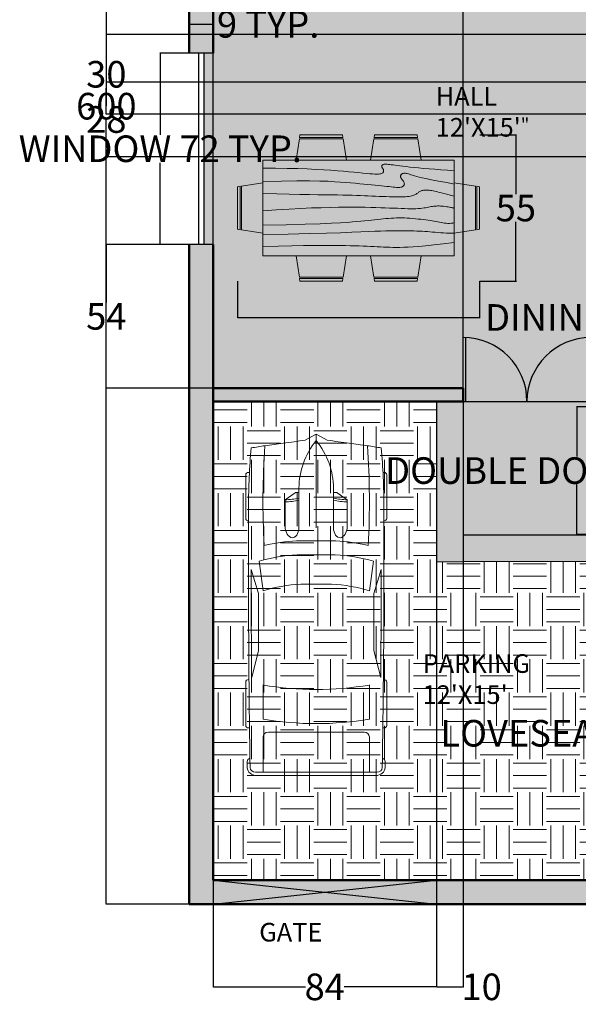
# Model space of a CAD drawing. Units: inches. Extents: x 77 to 548, y 631 to 1307.
# Tile 1 of 4: x 77 to 287, y 631 to 1001. Entities that reach past the tile are written whole.
import ezdxf

# ---------------------------------------------------------------- set-up
doc = ezdxf.new("R2010")
doc.units = ezdxf.units.IN
doc.header["$MEASUREMENT"] = 0
for name, color, linetype, lineweight in [('A-ANNO-DIMS', 2, 'Continuous', 18), ('A-ANNO-TEXT', 7, 'Continuous', 18), ('A-AREA-IDEN', 7, 'Continuous', 18), ('A-FLOR-STRS', 7, 'Continuous', 25), ('A-SITE-GATE', 7, 'Continuous', 25), ('A-WALL', 7, 'Continuous', 50), ('CAR', 7, 'Continuous', 13), ('DOORS', 4, 'Continuous', 25), ('FURNITURE', 34, 'Continuous', 18), ('WINDOW', 6, 'Continuous', 25)]:
    doc.layers.add(name, color=color, linetype=linetype, lineweight=lineweight)
for name, color, linetype, lineweight, true_color in [('A-FLOR-PATT', 254, 'Continuous', 13, 0xd7ebd2), ('A-WALL-PATT', 252, 'Continuous', 13, 0x939598), ('C-PVMT-PATT', 31, 'Continuous', 13, 0xfecc66)]:
    doc.layers.add(name, color=color, linetype=linetype, lineweight=lineweight, true_color=true_color)
doc.styles.get("Standard").update_dxf_attribs({"font": 'arial.ttf'})
doc.dimstyles.get("Standard").update_dxf_attribs({"dimtxt": 10, "dimasz": 0.18, "dimexe": 0.18, "dimexo": 0.0625, "dimgap": 0.09, "dimtad": 0, "dimtih": 1, "dimtoh": 1, "dimdec": 0, "dimzin": 0, "dimdsep": 46, "dimlunit": 3, "dimtxsty": 'Standard', "dimcen": 0.09, "dimadec": 0, "dimazin": 0, "dimtfac": 1, "dimtdec": 0, "dimtofl": 0, "dimtmove": 0, "dimatfit": 3, "dimfxl": 1, "dimtolj": 1, "dimtzin": 0, "dimarcsym": 0})

# ---------------------------------------------------------------- blocks, each defined once
blk = doc.blocks.new('*U3')
for p, q in [((46.55, 38.89), (22.35, 38.89)), ((136.7, 38.89), (160.9, 38.89)), ((21.1, 37.41), (21.1, 36.83)), ((47.8, 37.39), (47.8, 37.41)), ((87.99, 31.87), (74.76, 35.92)), ((134.31, 35.6), (119.29, 31.78)), ((135.45, 37.07), (135.45, 37.41)), ((162.15, 37.41), (162.15, 36.77)), ((186.47, -33.5), (186.47, 33.5)), ((188.4, -32.76), (188.4, 32.76)), ((70.03, 31.54), (86.41, 29.35)), ((138.42, 29.35), (157.25, 29.35)), ((186.47, 29.35), (167.01, 29.35)), ((164.52, 26.39), (164.52, -26.39)), ((32.27, 11.63), (36.13, 17.17)), ((36.13, 17.17), (50.94, 17.17)), ((32.12, 9.51), (32.12, 11.15)), ((3.27, 6.13), (0.1, 0.41)), ((29.77, 9.51), (51.68, 9.51)), ((58.92, -10.77), (58.92, 10.77)), ((66.55, -10.53), (66.55, 10.53)), ((82.74, 8.5), (82.74, -8.5)), ((186.47, -10.53), (186.47, 10.53)), ((0, 0), (51.68, 0)), ((0.1, -0.41), (3.27, -6.13)), ((29.77, -9.51), (51.68, -9.51)), ((32.12, -9.51), (32.12, -11.15)), ((32.27, -11.63), (36.13, -17.17)), ((36.13, -17.17), (50.94, -17.17)), ((86.41, -29.35), (70.03, -31.54)), ((87.99, -31.87), (74.76, -35.92)), ((134.31, -35.6), (119.29, -31.78)), ((157.25, -29.35), (138.42, -29.35)), ((167.01, -29.35), (186.47, -29.35)), ((21.1, -37.41), (21.1, -36.83)), ((47.8, -37.39), (47.8, -37.41)), ((135.45, -37.07), (135.45, -37.41)), ((162.15, -37.41), (162.15, -36.77)), ((46.55, -38.89), (22.35, -38.89)), ((136.7, -38.89), (160.9, -38.89))]:
    blk.add_line(p, q)
for centre, major_axis, ratio, start_param, end_param in [((22.35, 37.41), (0, -1.48), 0.842304, 3.141593, 4.712389), ((46.55, 37.41), (0, 1.48), 0.842304, -1.570796, 0), ((136.7, 37.41), (0, -1.48), 0.842304, 3.141593, 4.712389), ((160.9, 37.41), (0, 1.48), 0.842304, -1.570796, 0), ((180.63, 35.84), (0, 2.22), 0.842304, -0.013017, 1.249894), ((64.48, -10556.36), (0, 10595.31), 0.842304, -0.013397, -0.013017), ((266.03, -27.52), (0, 313.31), 0.842304, 1.367076, 1.39176), ((41.19, -490.86), (0, 528.23), 0.842304, 0.00281, 0.075598), ((64.48, -10555.62), (0, 10593.03), 0.842304, -0.013397, 0.002797), ((64.48, -10555.62), (0, -10591.55), 0.842304, 3.133765, 3.140441), ((183.98, 33.5), (0, -2.96), 0.842304, 1.570796, 3.128196), ((183.98, 32.76), (0, -5.25), 0.842304, 1.570796, 3.128196), ((259.18, -27.52), (0, -305.3), 0.842304, 4.528606, 4.561838), ((37.47, -593.96), (0, -623.33), 0.842304, 3.096046, 3.200911), ((134.4, 5.39), (0, -89.78), 0.842304, 4.449482, 4.652344), ((135.29, 5.39), (0, 81.77), 0.842304, 1.245306, 1.50788), ((149.6, 2.8), (0, -79.58), 0.842304, 4.372215, 4.640744), ((95.79, -3666.35), (0, -3698.24), 0.842304, 3.134049, 3.144098), ((17.08, 0), (0, 147.02), 0.842304, 4.511394, 4.913384), ((35.91, 0), (0, 147.02), 0.842304, 4.511394, 4.913384), ((167.01, 26.39), (0, 2.96), 0.842304, 0, 1.570796), ((-204.49, 52.4), (0, -250.96), 0.842304, 1.385369, 1.434372), ((13.04, 17.01), (0, 27.42), 0.842304, 4.435146, 4.718221), ((14.2, 17.01), (0, 27.42), 0.842304, 4.435146, 4.718221), ((50.79, 13.34), (6.34, -0.36), 0.603834, -1.395552, 1.581315), ((32.75, 11.15), (0, 0.74), 0.842304, 0.879714, 1.570796), ((29.77, -46.66), (0, 56.17), 0.842304, 0, 0.590319), ((0.62, 0), (0, -0.74), 0.842304, 4.131459, 5.293319), ((29.77, 46.66), (0, 56.17), 0.842304, 2.551274, 3.141593), ((-204.49, -52.4), (0, 250.96), 0.842304, -1.434372, -1.385369), ((13.04, -17.01), (0, -27.42), 0.842304, 1.564964, 1.848039), ((14.2, -17.01), (0, -27.42), 0.842304, 1.564964, 1.848039), ((134.4, -5.39), (0, -89.78), 0.842304, -1.510751, -1.307889), ((135.29, -5.39), (0, -81.77), 0.842304, -1.50788, -1.245306), ((149.6, -2.8), (0, -79.58), 0.842304, -1.499151, -1.230623), ((32.75, -11.15), (0, -0.74), 0.842304, 4.712389, 5.403472), ((259.18, 27.52), (0, 305.3), 0.842304, 1.721348, 1.754579), ((167.01, -26.39), (0, -2.96), 0.842304, 4.712389, 6.283185), ((266.03, 27.52), (0, 313.31), 0.842304, 1.749832, 1.774517), ((37.47, 593.96), (0, -623.33), 0.842304, -0.059319, 0.045547), ((95.79, 3666.35), (0, -3698.24), 0.842304, -0.002505, 0.007544), ((41.19, 490.86), (0, -528.23), 0.842304, -0.075598, -0.00281), ((22.35, -37.41), (0, 1.48), 0.842304, 1.570796, 3.141593), ((64.48, 10555.62), (0, 10593.03), 0.842304, 3.138796, 3.15499), ((46.55, -37.41), (0, -1.48), 0.842304, 0, 1.570796), ((64.48, 10555.62), (0, -10591.55), 0.842304, 0.001152, 0.007828), ((136.7, -37.41), (0, -1.48), 0.842304, -1.570796, 0), ((160.9, -37.41), (0, 1.48), 0.842304, 3.141593, 4.712389), ((180.63, -35.84), (0, -2.22), 0.842304, -1.249894, 0.013017), ((64.48, 10556.36), (0, 10595.31), 0.842304, 3.15461, 3.15499), ((183.98, -33.5), (0, 2.96), 0.842304, 3.15499, 4.712389), ((183.98, -32.76), (0, -5.25), 0.842304, 0.013397, 1.570796)]:
    blk.add_ellipse(centre, major_axis=major_axis, ratio=ratio, start_param=start_param, end_param=end_param)
at = {"extrusion": (0, 0, -1)}
blk.add_ellipse((50.79, -13.34), major_axis=(6.34, 0.36), ratio=0.603834, start_param=-1.395552, end_param=1.581315, dxfattribs=at)
blk = doc.blocks.new('Dining Set - 36 x 72 in.')
for p, q in [((-22.2343, 26.00059), (-23.4847, 17.99762)), ((-22.2304, 26), (-5.7608, 26)), ((-22, 27.5), (-22.1562, 26.50042)), ((-5.8416, 26.5), (-22.1534, 26.5)), ((-22, 27.5), (-6, 27.5)), ((-5.8437, 26.49966), (-6, 27.5)), ((-4.5152, 17.99762), (-5.7655, 25.99926)), ((5.7657, 26.00059), (4.5153, 17.99762)), ((5.7696, 26), (22.2392, 26)), ((6, 27.5), (5.8438, 26.50042)), ((22.1584, 26.5), (5.8466, 26.5)), ((6, 27.5), (22, 27.5)), ((22.1563, 26.49966), (22, 27.5)), ((23.4848, 17.99762), (22.2345, 25.99926)), ((36, 18), (-36, 18)), ((-36, 18), (-36, -18)), ((36, -18), (36, 18)), ((-45.5, 8), (-44.5004, 8.15617)), ((-45.5, 8), (-45.5, -8)), ((-44.5, -8.15843), (-44.5, 8.15338)), ((-44.0006, 8.23428), (-35.9976, 9.48474)), ((-44, 8.23041), (-44, -8.23915)), ((44.0006, 8.23428), (35.9976, 9.48474)), ((44, 8.23041), (44, -8.23915)), ((44.5, -8.15843), (44.5, 8.15338)), ((45.5, 8), (44.5005, 8.15617)), ((45.5, 8), (45.5, -8)), ((-44.4997, -8.15631), (-45.5, -8)), ((-35.9976, -9.48476), (-43.9993, -8.2345)), ((35.9976, -9.48476), (43.9993, -8.2345)), ((44.4997, -8.15631), (45.5, -8)), ((-36, -18), (36, -18)), ((-22.2343, -26.0006), (-23.4847, -17.99762)), ((-4.5152, -17.99762), (-5.7655, -25.99928)), ((5.7657, -26.0006), (4.5153, -17.99762)), ((23.4848, -17.99762), (22.2345, -25.99928)), ((-22.2304, -26), (-5.7608, -26)), ((-22, -27.5), (-22.1562, -26.50044)), ((-5.8416, -26.5), (-22.1534, -26.5)), ((-22, -27.5), (-6, -27.5)), ((-5.8437, -26.49967), (-6, -27.5)), ((5.7696, -26), (22.2392, -26)), ((6, -27.5), (5.8438, -26.50044)), ((22.1584, -26.5), (5.8466, -26.5)), ((6, -27.5), (22, -27.5)), ((22.1563, -26.49967), (22, -27.5))]:
    blk.add_line(p, q)
for points in [[(-36, 15), (-31.1772, 14.97754), (-26.8079, 14.91406), (-22.8538, 14.81543), (-19.276, 14.6875), (-16.0362, 14.53613), (-13.0957, 14.36718), (-10.4159, 14.18652), (-7.9583, 14), (-5.6904, 13.81315), (-3.6035, 13.63021), (-1.6954, 13.45508), (0.0365, 13.29166), (1.5945, 13.14388), (2.9811, 13.01562), (4.1988, 12.9108), (5.25, 12.83333), (6.1393, 12.78613), (6.8802, 12.76823), (7.4883, 12.77767), (7.9792, 12.8125), (8.3685, 12.87077), (8.6719, 12.95052), (8.9049, 13.0498), (9.0833, 13.16666), (9.2205, 13.29899), (9.3216, 13.44401), (9.3895, 13.59879), (9.4271, 13.76041), (9.4373, 13.92594), (9.4232, 14.09245), (9.3875, 14.257), (9.3333, 14.41666), (9.2638, 14.56917), (9.1836, 14.71484), (9.0975, 14.85465), (9.0104, 14.98958), (8.9272, 15.1206), (8.8529, 15.2487), (8.7922, 15.37483), (8.75, 15.5), (8.7305, 15.62467), (8.7344, 15.74739), (8.7617, 15.86621), (8.8125, 15.97916), (8.8867, 16.08431), (8.9844, 16.17968), (9.1055, 16.26334), (9.25, 16.33333), (9.4189, 16.38802), (9.6172, 16.42708), (9.8506, 16.45052), (10.125, 16.45833), (10.4463, 16.45052), (10.8203, 16.42708), (11.2529, 16.38802), (11.75, 16.33333), (12.3184, 16.26318), (12.9694, 16.17838), (13.7151, 16.07991), (14.5677, 15.96875), (15.5395, 15.84586), (16.6426, 15.71224), (17.8893, 15.56884), (19.2917, 15.41666), (20.859, 15.25667), (22.5879, 15.08984), (24.4721, 14.91715), (26.5052, 14.73958), (28.6809, 14.5581), (30.9929, 14.3737), (33.4347, 14.18733), (36, 14)], [(-36, 10), (-28.9766, 10.14274), (-23.1725, 10.20442), (-18.4241, 10.19775), (-14.5677, 10.13541), (-11.4399, 10.03011), (-8.877, 9.89453), (-6.7154, 9.74137), (-4.7917, 9.58333), (-2.9698, 9.43082), (-1.2246, 9.28515), (0.4415, 9.14534), (2.026, 9.01041), (3.5266, 8.87939), (4.9408, 8.7513), (6.266, 8.62516), (7.5, 8.5), (8.6411, 8.37549), (9.6914, 8.2539), (10.6538, 8.13818), (11.5312, 8.03125), (12.3267, 7.93603), (13.043, 7.85547), (13.6831, 7.79248), (14.25, 7.75), (14.7471, 7.7303), (15.1797, 7.73307), (15.5537, 7.75732), (15.875, 7.80208), (16.1494, 7.86637), (16.3828, 7.94922), (16.5811, 8.04964), (16.75, 8.16666), (16.8944, 8.29915), (17.0143, 8.44531), (17.1089, 8.60319), (17.1771, 8.77083), (17.218, 8.94629), (17.2305, 9.1276), (17.2137, 9.31282), (17.1667, 9.5), (17.0895, 9.6875), (16.987, 9.875), (16.8649, 10.0625), (16.7292, 10.25), (16.5856, 10.4375), (16.4401, 10.625), (16.2985, 10.8125), (16.1667, 11), (16.05, 11.18733), (15.9518, 11.3737), (15.8752, 11.5581), (15.8229, 11.73958), (15.798, 11.91715), (15.8034, 12.08984), (15.842, 12.25667), (15.9167, 12.41666), (16.0295, 12.56836), (16.1784, 12.70833), (16.3605, 12.83268), (16.5729, 12.9375), (16.8127, 13.01888), (17.0768, 13.07291), (17.3625, 13.0957), (17.6667, 13.08333), (17.9894, 13.03312), (18.3418, 12.94726), (18.7382, 12.82918), (19.1927, 12.68229), (19.7195, 12.51001), (20.3327, 12.31575), (21.0465, 12.10294), (21.875, 11.875), (22.8357, 11.63354), (23.959, 11.37304), (25.2786, 11.08618), (26.8282, 10.76562), (28.6414, 10.40405), (30.752, 9.99414), (33.1936, 9.52856), (36, 9)], [(-36, 5.5), (-30.7157, 5.3348), (-26.069, 5.20963), (-21.9946, 5.11767), (-18.4271, 5.05208), (-15.3009, 5.00602), (-12.5508, 4.97265), (-10.1112, 4.94515), (-7.9167, 4.91666), (-5.909, 4.88167), (-4.0586, 4.83984), (-2.3429, 4.79215), (-0.7396, 4.73958), (0.7739, 4.6831), (2.22, 4.6237), (3.6213, 4.56233), (5, 4.5), (6.373, 4.43782), (7.7344, 4.3776), (9.0723, 4.32129), (10.375, 4.27083), (11.6309, 4.22819), (12.8281, 4.19531), (13.9551, 4.17415), (15, 4.16666), (15.954, 4.17448), (16.819, 4.19791), (17.6001, 4.23698), (18.3021, 4.29166), (18.9299, 4.36198), (19.4883, 4.44791), (19.9823, 4.54948), (20.4167, 4.66666), (20.7969, 4.79899), (21.1302, 4.94401), (21.4245, 5.09879), (21.6875, 5.26041), (21.9271, 5.42594), (22.1511, 5.59245), (22.3672, 5.757), (22.5834, 5.91666), (22.8065, 6.06868), (23.0404, 6.21093), (23.2879, 6.34147), (23.5521, 6.45833), (23.8358, 6.55957), (24.142, 6.64323), (24.4735, 6.70735), (24.8334, 6.75), (25.2235, 6.76969), (25.642, 6.76692), (26.0858, 6.74267), (26.5521, 6.69791), (27.0379, 6.63362), (27.5404, 6.55078), (28.0565, 6.45036), (28.5834, 6.33333), (29.1242, 6.19987), (29.7071, 6.04687), (30.3661, 5.87044), (31.1354, 5.66666), (32.0493, 5.43164), (33.142, 5.16146), (34.4475, 4.85221), (36, 4.5)], [(-36, -1), (-30.7915, -0.6591), (-26.0195, -0.38216), (-21.6519, -0.16284), (-17.6563, 0.00521), (-14.0005, 0.12833), (-10.6523, 0.21289), (-7.5796, 0.26522), (-4.75, 0.29166), (-2.134, 0.29793), (0.2878, 0.28711), (2.5317, 0.26163), (4.6146, 0.22396), (6.5529, 0.17651), (8.3633, 0.12174), (10.0623, 0.06209), (11.6667, 0), (13.1899, -0.06201), (14.6341, -0.1211), (15.9982, -0.17432), (17.2813, -0.21875), (18.4823, -0.25147), (19.6003, -0.26953), (20.6343, -0.27002), (21.5834, -0.25), (22.4481, -0.20768), (23.2357, -0.14584), (23.9549, -0.06836), (24.6146, 0.02083), (25.2235, 0.11784), (25.7904, 0.21875), (26.3241, 0.31966), (26.8334, 0.41666), (27.3265, 0.50618), (27.8099, 0.58593), (28.2894, 0.65397), (28.7709, 0.70833), (29.2601, 0.74707), (29.763, 0.76823), (30.2855, 0.76985), (30.8334, 0.75), (31.4088, 0.70784), (31.9994, 0.64713), (32.589, 0.57275), (33.1615, 0.48958), (33.7008, 0.4025), (34.1908, 0.3164), (34.6153, 0.23616), (34.9584, 0.16666), (35.2099, 0.11165), (35.3848, 0.07031), (35.504, 0.04069), (35.5886, 0.02083), (35.6594, 0.00879), (35.7377, 0.0026), (35.8442, 0.00032), (36, 0)], [(-36, -6.5), (-27.1843, -6.31267), (-20.084, -6.1263), (-14.469, -5.9419), (-10.1094, -5.76042), (-6.7752, -5.58285), (-4.2363, -5.41016), (-2.2629, -5.24333), (-0.625, -5.08334), (0.8708, -4.93099), (2.2715, -4.78646), (3.5872, -4.64974), (4.8281, -4.52084), (6.0046, -4.39974), (7.127, -4.28646), (8.2053, -4.18099), (9.25, -4.08334), (10.2705, -3.99382), (11.2734, -3.91407), (12.2647, -3.84603), (13.25, -3.79167), (14.2354, -3.75293), (15.2266, -3.73177), (16.2295, -3.73015), (17.25, -3.75), (18.2912, -3.79248), (19.3451, -3.85547), (20.4009, -3.93604), (21.4479, -4.03125), (22.4754, -4.13819), (23.4727, -4.25391), (24.4289, -4.37549), (25.3334, -4.5), (26.1785, -4.62492), (26.9694, -4.74935), (27.7145, -4.87281), (28.4219, -4.99479), (29.1, -5.11483), (29.7572, -5.23242), (30.4016, -5.34709), (31.0417, -5.45834), (31.6837, -5.56437), (32.3262, -5.65821), (32.9658, -5.73153), (33.599, -5.77604), (34.2224, -5.78345), (34.8327, -5.74545), (35.4264, -5.65373), (36, -5.5)], [(-36, -10), (-26.4022, -9.81299), (-18.4675, -9.62891), (-11.9839, -9.45069), (-6.7396, -9.28125), (-2.5226, -9.12354), (0.8789, -8.98047), (3.6769, -8.85498), (6.0833, -8.75), (8.2767, -8.66765), (10.3021, -8.60677), (12.1712, -8.56543), (13.8958, -8.54167), (15.4876, -8.53353), (16.9583, -8.53907), (18.3197, -8.55632), (19.5834, -8.58334), (20.7616, -8.61841), (21.8685, -8.66081), (22.9188, -8.71004), (23.9271, -8.76563), (24.9081, -8.82707), (25.8763, -8.89388), (26.8465, -8.96558), (27.8334, -9.04167), (28.8474, -9.12118), (29.8828, -9.20117), (30.93, -9.27824), (31.9792, -9.34896), (33.0205, -9.40991), (34.0443, -9.45768), (35.0407, -9.48885), (36, -9.5)], [(-36, -14.5), (-30.0881, -14.33513), (-25.0332, -14.21224), (-20.7312, -14.12647), (-17.0781, -14.07292), (-13.97, -14.04671), (-11.3027, -14.04297), (-8.9724, -14.05681), (-6.875, -14.08334), (-4.9224, -14.11833), (-3.0905, -14.16016), (-1.3709, -14.20785), (0.2448, -14.26042), (1.7647, -14.3169), (3.1973, -14.3763), (4.5507, -14.43767), (5.8333, -14.5), (7.0554, -14.5621), (8.235, -14.62175), (9.3922, -14.67652), (10.5469, -14.72396), (11.7192, -14.76164), (12.929, -14.78711), (14.1965, -14.79794), (15.5417, -14.79167), (16.9933, -14.76424), (18.6152, -14.70508), (20.4804, -14.60197), (22.6615, -14.44271), (25.2312, -14.21509), (28.2624, -13.9069), (31.8277, -13.50594), (36, -13)]]:
    blk.add_lwpolyline(points)
blk = doc.blocks.new('WINDOW-72')
for p, q in [((9, 72), (0, 72)), ((3.5, 72), (3.5, 0)), ((5.5, 72), (5.5, 0)), ((9, 0), (0, 0))]:
    blk.add_line(p, q)
blk = doc.blocks.new('DOOR-DOUBLE-48')
for p, q in [((0, 0), (0, 24)), ((1, 0), (1, 23.98)), ((47, 0), (47, 23.98)), ((48, 0), (48, 24)), ((0, 0), (1, 0)), ((47, 0), (48, 0))]:
    blk.add_line(p, q)
for centre, start, end in [((0, 0), 0, 90), ((48, 0), 90, 180)]:
    blk.add_arc(centre, 24, start, end)
blk = doc.blocks.new('*D24')
at = {"layer": 'A-ANNO-DIMS', "color": 0, "lineweight": -2, "transparency": 16777216}
for p, q in [((140.6, 988.89), (129.68, 988.89)), ((129.86, 988.71), (129.86, 958.15)), ((129.86, 917.07), (129.86, 947.62)), ((140.6, 916.89), (129.68, 916.89))]:
    blk.add_line(p, q, dxfattribs=at)
at = {"layer": 'A-ANNO-DIMS', "color": 0, "transparency": 16777216}
for points in [[(129.83, 988.71), (129.89, 988.71), (129.86, 988.89)], [(129.83, 917.07), (129.89, 917.07), (129.86, 916.89)]]:
    blk.add_solid(points, dxfattribs=at)
at = {"layer": 'Defpoints', "color": 0, "transparency": 16777216}
for p in [(129.86, 988.89), (140.66, 988.89), (140.66, 916.89)]:
    blk.add_point(p, dxfattribs=at)
at = {"layer": 'A-ANNO-DIMS', "color": 0, "transparency": 16777216, "insert": (129.86, 952.89), "char_height": 10, "attachment_point": 5}
blk.add_mtext('\\A1;WINDOW 72 TYP.', dxfattribs=at)
blk = doc.blocks.new('*D25')
at = {"layer": 'A-ANNO-DIMS', "color": 0, "lineweight": -2, "transparency": 16777216}
for p, q in [((140.66, 988.95), (140.66, 999.87)), ((140.84, 999.69), (149.48, 999.69)), ((149.66, 988.95), (149.66, 999.87)), ((149.66, 999.69), (149.84, 999.69))]:
    blk.add_line(p, q, dxfattribs=at)
at = {"layer": 'A-ANNO-DIMS', "color": 0, "transparency": 16777216}
for points in [[(140.84, 999.72), (140.84, 999.66), (140.66, 999.69)], [(149.48, 999.72), (149.48, 999.66), (149.66, 999.69)]]:
    blk.add_solid(points, dxfattribs=at)
at = {"layer": 'Defpoints', "color": 0, "transparency": 16777216}
for p in [(149.66, 999.69), (140.66, 988.89), (149.66, 988.89)]:
    blk.add_point(p, dxfattribs=at)
at = {"layer": 'A-ANNO-DIMS', "color": 0, "transparency": 16777216, "insert": (170.39, 999.69), "char_height": 10, "attachment_point": 5}
blk.add_mtext('\\A1;9 TYP.', dxfattribs=at)
blk = doc.blocks.new('*D26')
at = {"layer": 'A-ANNO-DIMS', "color": 0, "lineweight": -2, "transparency": 16777216}
for p, q in [((293.6, 855.89), (286.28, 855.89)), ((286.46, 855.71), (286.46, 837.15)), ((286.46, 808.07), (286.46, 826.62)), ((293.6, 807.89), (286.28, 807.89))]:
    blk.add_line(p, q, dxfattribs=at)
at = {"layer": 'A-ANNO-DIMS', "color": 0, "transparency": 16777216}
for points in [[(286.43, 855.71), (286.49, 855.71), (286.46, 855.89)], [(286.43, 808.07), (286.49, 808.07), (286.46, 807.89)]]:
    blk.add_solid(points, dxfattribs=at)
at = {"layer": 'Defpoints', "color": 0, "transparency": 16777216}
for p in [(293.66, 855.89), (286.46, 807.89), (293.66, 807.89)]:
    blk.add_point(p, dxfattribs=at)
at = {"layer": 'A-ANNO-DIMS', "color": 0, "transparency": 16777216, "insert": (286.46, 831.89), "char_height": 10, "attachment_point": 5}
blk.add_mtext('\\A1;DOUBLE DOOR 48 TYP.', dxfattribs=at)
blk = doc.blocks.new('*D36')
at = {"layer": 'A-ANNO-DIMS', "color": 0, "lineweight": -2, "transparency": 16777216}
for p, q in [((158.85, 903.05), (158.85, 889.28)), ((249.85, 903.05), (249.85, 889.28)), ((159.03, 889.46), (249.67, 889.46)), ((249.85, 889.46), (250.03, 889.46))]:
    blk.add_line(p, q, dxfattribs=at)
at = {"layer": 'A-ANNO-DIMS', "color": 0, "transparency": 16777216}
for points in [[(159.03, 889.49), (159.03, 889.43), (158.85, 889.46)], [(249.67, 889.49), (249.67, 889.43), (249.85, 889.46)]]:
    blk.add_solid(points, dxfattribs=at)
at = {"layer": 'Defpoints', "color": 0, "transparency": 16777216}
for p in [(158.85, 903.11), (249.85, 903.11), (249.85, 889.46)]:
    blk.add_point(p, dxfattribs=at)
at = {"layer": 'A-ANNO-DIMS', "color": 0, "transparency": 16777216, "insert": (297.98, 889.46), "char_height": 10, "attachment_point": 5}
blk.add_mtext('\\A1;DINING SET 91', dxfattribs=at)
blk = doc.blocks.new('*D37')
at = {"layer": 'A-ANNO-DIMS', "color": 0, "lineweight": -2, "transparency": 16777216}
for p, q in [((249.91, 958.11), (263.68, 958.11)), ((263.5, 957.93), (263.5, 935.79)), ((263.5, 903.29), (263.5, 925.44)), ((249.91, 903.11), (263.68, 903.11))]:
    blk.add_line(p, q, dxfattribs=at)
at = {"layer": 'A-ANNO-DIMS', "color": 0, "transparency": 16777216}
for points in [[(263.47, 957.93), (263.53, 957.93), (263.5, 958.11)], [(263.47, 903.29), (263.53, 903.29), (263.5, 903.11)]]:
    blk.add_solid(points, dxfattribs=at)
at = {"layer": 'Defpoints', "color": 0, "transparency": 16777216}
for p in [(249.85, 958.11), (263.5, 958.11), (249.85, 903.11)]:
    blk.add_point(p, dxfattribs=at)
at = {"layer": 'A-ANNO-DIMS', "color": 0, "transparency": 16777216, "insert": (263.5, 930.61), "char_height": 10, "attachment_point": 5}
blk.add_mtext('\\A1;55', dxfattribs=at)
blk = doc.blocks.new('*D40')
at = {"layer": 'A-ANNO-DIMS', "color": 0, "lineweight": -2, "transparency": 16777216}
for p, q in [((323.26, 733.13), (323.08, 733.13)), ((323.26, 724.2), (323.26, 733.31)), ((383.08, 733.13), (323.44, 733.13)), ((383.26, 724.2), (383.26, 733.31))]:
    blk.add_line(p, q, dxfattribs=at)
at = {"layer": 'A-ANNO-DIMS', "color": 0, "transparency": 16777216}
for points in [[(323.44, 733.16), (323.44, 733.1), (323.26, 733.13)], [(383.08, 733.16), (383.08, 733.1), (383.26, 733.13)]]:
    blk.add_solid(points, dxfattribs=at)
at = {"layer": 'Defpoints', "color": 0, "transparency": 16777216}
for p in [(323.26, 733.13), (323.26, 724.13), (383.26, 724.13)]:
    blk.add_point(p, dxfattribs=at)
at = {"layer": 'A-ANNO-DIMS', "color": 0, "transparency": 16777216, "insert": (277.25, 733.13), "char_height": 10, "attachment_point": 5}
blk.add_mtext('\\A1;LOVESEAT 60', dxfattribs=at)
blk = doc.blocks.new('*D43')
at = {"layer": 'A-ANNO-DIMS', "color": 0, "lineweight": -2, "transparency": 16777216}
for p, q in [((140.6, 1268.89), (109.38, 1268.89)), ((109.56, 1268.71), (109.56, 974.08)), ((109.56, 669.07), (109.56, 963.69)), ((140.6, 668.89), (109.38, 668.89))]:
    blk.add_line(p, q, dxfattribs=at)
at = {"layer": 'A-ANNO-DIMS', "color": 0, "transparency": 16777216}
for points in [[(109.53, 1268.71), (109.59, 1268.71), (109.56, 1268.89)], [(109.53, 669.07), (109.59, 669.07), (109.56, 668.89)]]:
    blk.add_solid(points, dxfattribs=at)
at = {"layer": 'Defpoints', "color": 0, "transparency": 16777216}
for p in [(109.56, 1268.89), (140.66, 1268.89), (140.66, 668.89)]:
    blk.add_point(p, dxfattribs=at)
at = {"layer": 'A-ANNO-DIMS', "color": 0, "transparency": 16777216, "insert": (109.56, 968.89), "char_height": 10, "attachment_point": 5}
blk.add_mtext('\\A1;600', dxfattribs=at)
blk = doc.blocks.new('*D44')
at = {"layer": 'A-ANNO-DIMS', "color": 0, "lineweight": -2, "transparency": 16777216}
for p, q in [((149.66, 668.83), (149.66, 637.61)), ((233.66, 668.83), (233.66, 637.61)), ((149.84, 637.79), (184.42, 637.79)), ((233.48, 637.79), (198.9, 637.79))]:
    blk.add_line(p, q, dxfattribs=at)
at = {"layer": 'A-ANNO-DIMS', "color": 0, "transparency": 16777216}
for points in [[(149.84, 637.82), (149.84, 637.76), (149.66, 637.79)], [(233.48, 637.82), (233.48, 637.76), (233.66, 637.79)]]:
    blk.add_solid(points, dxfattribs=at)
at = {"layer": 'Defpoints', "color": 0, "transparency": 16777216}
for p in [(149.66, 668.89), (233.66, 668.89), (233.66, 637.79)]:
    blk.add_point(p, dxfattribs=at)
at = {"layer": 'A-ANNO-DIMS', "color": 0, "transparency": 16777216, "insert": (191.66, 637.79), "char_height": 10, "attachment_point": 5}
blk.add_mtext('\\A1;84', dxfattribs=at)
blk = doc.blocks.new('*D47')
at = {"layer": 'A-ANNO-DIMS', "color": 0, "lineweight": -2, "transparency": 16777216}
for p, q in [((140.6, 916.89), (109.38, 916.89)), ((109.56, 916.71), (109.56, 895.06)), ((109.56, 863.07), (109.56, 884.71)), ((149.6, 862.89), (109.38, 862.89))]:
    blk.add_line(p, q, dxfattribs=at)
at = {"layer": 'A-ANNO-DIMS', "color": 0, "transparency": 16777216}
for points in [[(109.53, 916.71), (109.59, 916.71), (109.56, 916.89)], [(109.53, 863.07), (109.59, 863.07), (109.56, 862.89)]]:
    blk.add_solid(points, dxfattribs=at)
at = {"layer": 'Defpoints', "color": 0, "transparency": 16777216}
for p in [(140.66, 916.89), (109.56, 862.89), (149.66, 862.89)]:
    blk.add_point(p, dxfattribs=at)
at = {"layer": 'A-ANNO-DIMS', "color": 0, "transparency": 16777216, "insert": (109.56, 889.89), "char_height": 10, "attachment_point": 5}
blk.add_mtext('\\A1;54', dxfattribs=at)
blk = doc.blocks.new('*D54')
at = {"layer": 'A-ANNO-DIMS', "color": 0, "lineweight": -2, "transparency": 16777216}
for p, q in [((351.6, 995.89), (109.38, 995.89)), ((109.56, 995.71), (109.56, 986.09)), ((109.56, 966.07), (109.56, 975.69)), ((351.6, 965.89), (109.38, 965.89))]:
    blk.add_line(p, q, dxfattribs=at)
at = {"layer": 'A-ANNO-DIMS', "color": 0, "transparency": 16777216}
for points in [[(109.53, 995.71), (109.59, 995.71), (109.56, 995.89)], [(109.53, 966.07), (109.59, 966.07), (109.56, 965.89)]]:
    blk.add_solid(points, dxfattribs=at)
at = {"layer": 'Defpoints', "color": 0, "transparency": 16777216}
for p in [(109.56, 995.89), (351.66, 995.89), (351.66, 965.89)]:
    blk.add_point(p, dxfattribs=at)
at = {"layer": 'A-ANNO-DIMS', "color": 0, "transparency": 16777216, "insert": (109.56, 980.89), "char_height": 10, "attachment_point": 5}
blk.add_mtext('\\A1;30', dxfattribs=at)
blk = doc.blocks.new('*D56')
at = {"layer": 'A-ANNO-DIMS', "color": 0, "lineweight": -2, "transparency": 16777216}
for p, q in [((149.66, 857.95), (149.66, 1300.17)), ((149.84, 1299.99), (189.43, 1299.99)), ((243.48, 1299.99), (203.89, 1299.99)), ((243.66, 857.95), (243.66, 1300.17))]:
    blk.add_line(p, q, dxfattribs=at)
at = {"layer": 'A-ANNO-DIMS', "color": 0, "transparency": 16777216}
for points in [[(149.84, 1300.02), (149.84, 1299.96), (149.66, 1299.99)], [(243.48, 1300.02), (243.48, 1299.96), (243.66, 1299.99)]]:
    blk.add_solid(points, dxfattribs=at)
at = {"layer": 'Defpoints', "color": 0, "transparency": 16777216}
for p in [(243.66, 1299.99), (149.66, 857.89), (243.66, 857.89)]:
    blk.add_point(p, dxfattribs=at)
at = {"layer": 'A-ANNO-DIMS', "color": 0, "transparency": 16777216, "insert": (196.66, 1299.99), "char_height": 10, "attachment_point": 5}
blk.add_mtext('\\A1;94', dxfattribs=at)
blk = doc.blocks.new('*D59')
at = {"layer": 'A-ANNO-DIMS', "color": 0, "lineweight": -2, "transparency": 16777216}
for p, q in [((385.62, 977.89), (109.38, 977.89)), ((109.56, 977.71), (109.56, 969.08)), ((109.56, 950.07), (109.56, 958.69)), ((375.12, 949.89), (109.38, 949.89))]:
    blk.add_line(p, q, dxfattribs=at)
at = {"layer": 'A-ANNO-DIMS', "color": 0, "transparency": 16777216}
for points in [[(109.53, 977.71), (109.59, 977.71), (109.56, 977.89)], [(109.53, 950.07), (109.59, 950.07), (109.56, 949.89)]]:
    blk.add_solid(points, dxfattribs=at)
at = {"layer": 'Defpoints', "color": 0, "transparency": 16777216}
for p in [(109.56, 977.89), (385.68, 977.89), (375.18, 949.89)]:
    blk.add_point(p, dxfattribs=at)
at = {"layer": 'A-ANNO-DIMS', "color": 0, "transparency": 16777216, "insert": (109.56, 963.89), "char_height": 10, "attachment_point": 5}
blk.add_mtext('\\A1;28', dxfattribs=at)
blk = doc.blocks.new('*D61')
at = {"layer": 'A-ANNO-DIMS', "color": 0, "lineweight": -2, "transparency": 16777216}
for p, q in [((243.66, 807.62), (243.66, 637.61)), ((233.66, 797.58), (233.66, 637.61)), ((233.84, 637.79), (243.48, 637.79)), ((243.66, 637.79), (243.84, 637.79))]:
    blk.add_line(p, q, dxfattribs=at)
at = {"layer": 'A-ANNO-DIMS', "color": 0, "transparency": 16777216}
for points in [[(233.84, 637.82), (233.84, 637.76), (233.66, 637.79)], [(243.48, 637.82), (243.48, 637.76), (243.66, 637.79)]]:
    blk.add_solid(points, dxfattribs=at)
at = {"layer": 'Defpoints', "color": 0, "transparency": 16777216}
for p in [(243.66, 807.68), (233.66, 797.64), (243.66, 637.79)]:
    blk.add_point(p, dxfattribs=at)
at = {"layer": 'A-ANNO-DIMS', "color": 0, "transparency": 16777216, "insert": (250.61, 637.79), "char_height": 10, "attachment_point": 5}
blk.add_mtext('\\A1;10', dxfattribs=at)
blk = doc.blocks.new('*D62')
at = {"layer": 'A-ANNO-DIMS', "color": 0, "lineweight": -2, "transparency": 16777216}
for p, q in [((243.73, 857.89), (471.94, 857.89)), ((471.76, 857.71), (471.76, 837.98)), ((471.76, 807.86), (471.76, 827.59)), ((243.73, 807.68), (471.94, 807.68))]:
    blk.add_line(p, q, dxfattribs=at)
at = {"layer": 'A-ANNO-DIMS', "color": 0, "transparency": 16777216}
for points in [[(471.73, 857.71), (471.79, 857.71), (471.76, 857.89)], [(471.73, 807.86), (471.79, 807.86), (471.76, 807.68)]]:
    blk.add_solid(points, dxfattribs=at)
at = {"layer": 'Defpoints', "color": 0, "transparency": 16777216}
for p in [(243.66, 857.89), (471.76, 857.89), (243.66, 807.68)]:
    blk.add_point(p, dxfattribs=at)
at = {"layer": 'A-ANNO-DIMS', "color": 0, "transparency": 16777216, "insert": (471.76, 832.79), "char_height": 10, "attachment_point": 5}
blk.add_mtext('\\A1;50.2', dxfattribs=at)

msp = doc.modelspace()

# ---------------------------------------------------------------- hatches: boundary and pattern name
at = {"layer": 'A-FLOR-PATT'}
h = msp.add_hatch(color=256, dxfattribs=at)
h.dxf.hatch_style = 1
h.paths.add_polyline_path([(293.663, 1206.888), (291.663, 1206.888), (291.663, 1211.888), (293.663, 1211.888), (293.663, 1259.888), (149.663, 1259.888), (149.663, 1211.888), (257.663, 1211.888), (257.663, 1206.888), (245.663, 1206.888), (245.663, 1204.888), (245.663, 1174.888), (245.663, 1153.888), (149.663, 1153.888), (149.663, 1047.888), (255.663, 1047.888), (255.663, 1042.888), (149.663, 1042.888), (149.663, 988.888), (146.163, 988.888), (146.163, 916.888), (149.663, 916.888), (149.663, 862.888), (243.663, 862.888), (243.663, 857.888), (243.663, 807.683), (293.663, 807.888), (298.663, 807.888), (298.663, 677.888), (431.663, 677.888), (431.663, 702.459), (435.163, 702.459), (435.163, 774.459), (431.663, 774.459), (431.663, 857.888), (330.663, 857.888), (330.663, 862.888), (325.663, 944.888), (325.663, 949.888), (346.663, 949.888), (346.663, 965.888), (346.663, 995.888), (346.663, 997.888), (293.663, 997.888), (293.663, 1002.888), (293.663, 1004.888), (298.663, 1004.888), (298.663, 1002.888), (431.663, 1002.888), (431.663, 1095.888), (431.663, 1100.888), (431.663, 1147.888), (342.663, 1147.888), (342.663, 1174.888), (342.663, 1204.888), (342.663, 1206.888), (334.663, 1206.888), (334.663, 1211.888), (431.663, 1211.888), (431.663, 1259.888), (298.663, 1259.888), (298.663, 1211.888), (300.663, 1211.888), (300.663, 1206.888), (298.663, 1206.888), (298.663, 1042.888), (298.663, 1040.888), (293.663, 1040.888), (291.663, 1040.888), (291.663, 1047.888), (293.663, 1047.888)])
h.paths.add_polyline_path([(291.663, 862.888), (293.663, 862.888), (298.663, 862.888), (300.663, 862.888), (300.663, 857.888), (298.663, 857.888), (298.663, 855.888), (293.663, 855.888), (293.663, 857.888), (291.663, 857.888)], flags=16)
h.paths.add_polyline_path([(407.663, 920.888), (346.988, 920.888), (346.988, 944.888), (325.663, 944.888), (330.663, 862.888), (407.663, 862.888)], flags=17)
h.paths.add_polyline_path([(435.163, 988.679), (431.663, 988.679), (431.663, 997.888), (351.663, 997.888), (351.663, 995.888), (346.663, 995.888), (346.663, 965.888), (351.663, 965.888), (351.663, 949.888), (375.18, 949.888), (375.18, 957.888), (381.68, 957.888), (379.68, 963.887, -0.7025712), (385.68, 977.887, -0.7025621), (391.68, 963.888), (389.68, 957.888), (392.68, 957.888), (392.68, 959.388), (395.68, 959.388), (395.68, 957.888), (396.18, 957.888), (396.18, 949.888), (431.663, 949.888), (431.663, 964.679), (435.163, 964.679)])
h.paths.add_polyline_path([(431.663, 1206.888), (347.663, 1206.888), (347.663, 1204.888), (342.663, 1204.888), (342.663, 1174.888), (347.663, 1174.888), (347.663, 1167.048), (372.327, 1167.048), (372.327, 1152.888), (374.776, 1152.888), (374.776, 1160.888), (381.276, 1160.888), (379.276, 1166.887, -0.7025712), (385.276, 1180.887, -0.7025621), (391.276, 1166.888), (389.276, 1160.888), (392.276, 1160.888), (392.276, 1162.388), (395.276, 1162.388), (395.276, 1160.888), (395.776, 1160.888), (395.776, 1152.888), (431.663, 1152.888), (431.663, 1170.888), (435.163, 1170.888), (435.163, 1194.888), (431.663, 1194.888)])
h.paths.add_polyline_path([(245.663, 1204.888), (240.663, 1204.888), (240.663, 1206.888), (149.663, 1206.888), (149.663, 1194.888), (146.163, 1194.888), (146.163, 1170.888), (149.663, 1170.888), (149.663, 1158.888), (188.741, 1158.888), (188.741, 1166.888), (195.241, 1166.888), (193.241, 1172.887, -0.7025712), (199.241, 1186.887, -0.7025621), (205.241, 1172.888), (203.241, 1166.888), (206.241, 1166.888), (206.241, 1168.388), (209.241, 1168.388), (209.241, 1166.888), (209.741, 1166.888), (209.741, 1158.888), (215.999, 1158.888), (215.999, 1173.048), (240.663, 1173.048), (240.663, 1174.888), (245.663, 1174.888)], flags=17)
at = {"layer": 'A-WALL-PATT'}
h = msp.add_hatch(color=256, dxfattribs=at)
h.dxf.hatch_style = 1
h.paths.add_polyline_path([(149.663, 1042.888), (149.663, 1170.888), (140.663, 1170.888), (140.663, 988.888), (149.663, 988.888)])
h.paths.add_polyline_path([(149.663, 1259.888), (431.663, 1259.888), (431.663, 1194.888), (440.663, 1194.888), (440.663, 1268.888), (140.663, 1268.888), (140.663, 1194.888), (149.663, 1194.888), (149.663, 1206.888)])
h.paths.add_polyline_path([(298.663, 1259.888), (293.663, 1259.888), (293.663, 1211.888), (291.663, 1211.888), (291.663, 1206.888), (293.663, 1206.888), (293.663, 1047.888), (291.663, 1047.888), (291.663, 1040.888), (293.663, 1040.888), (298.663, 1040.888), (298.663, 1095.888), (298.663, 1206.888), (300.663, 1206.888), (300.663, 1211.888), (298.663, 1211.888)])
h.paths.add_polyline_path([(257.663, 1211.888), (149.663, 1211.888), (149.663, 1206.888), (240.663, 1206.888), (240.663, 1204.888), (241.135, 1204.888), (245.663, 1204.888), (245.663, 1206.888), (257.663, 1206.888)], flags=17)
h.paths.add_polyline_path([(431.663, 1211.888), (334.663, 1211.888), (334.663, 1206.888), (342.663, 1206.888), (342.663, 1204.888), (347.191, 1204.888), (347.663, 1204.888), (347.663, 1206.888), (431.663, 1206.888)], flags=17)
h.paths.add_polyline_path([(440.663, 1170.888), (431.663, 1170.888), (431.663, 1100.888), (431.663, 1047.888), (431.663, 988.679), (440.663, 988.679)])
h.paths.add_polyline_path([(431.663, 1002.888), (298.663, 1002.888), (298.663, 1004.888), (293.663, 1004.888), (293.663, 1002.888), (293.663, 997.888), (346.663, 997.888), (346.663, 995.888), (351.663, 995.888), (351.663, 997.888), (431.663, 997.888)])
h.paths.add_polyline_path([(440.663, 964.679), (431.663, 964.679), (431.663, 949.888), (351.663, 949.888), (351.663, 965.888), (346.663, 965.888), (346.663, 949.888), (325.663, 949.888), (325.663, 944.888), (431.663, 944.888), (431.663, 915.45), (440.663, 915.45)])
h.paths.add_polyline_path([(440.663, 891.45), (431.663, 891.45), (431.663, 862.888), (330.663, 862.888), (330.663, 857.888), (431.663, 857.888), (431.663, 774.459), (440.663, 774.459)], flags=17)
h.paths.add_polyline_path([(440.663, 702.459), (431.663, 702.459), (431.663, 677.888), (149.663, 677.888), (149.663, 916.888), (140.663, 916.888), (140.663, 668.888), (440.663, 668.888)])
h.paths.add_polyline_path([(293.663, 807.888), (243.663, 807.683), (243.663, 857.888), (233.663, 857.888), (233.663, 807.683), (233.663, 797.642), (243.704, 797.683), (293.663, 797.887)], flags=17)
h.paths.add_polyline_path([(243.663, 862.888), (149.663, 862.888), (149.663, 857.888), (243.663, 857.888)], flags=17)
at = {"layer": 'C-PVMT-PATT'}
h = msp.add_hatch(dxfattribs=at)
h.set_pattern_fill('EARTH', color=256, scale=50)
h.paths.add_polyline_path([(293.663, 797.887), (243.704, 797.683), (233.663, 797.642), (233.663, 807.683), (233.663, 857.888), (149.663, 857.888), (149.663, 677.888), (293.663, 677.888)])

# ---------------------------------------------------------------- linework, layer by layer
at = {"layer": 'A-FLOR-STRS'}
for p, q in [((233.663, 857.888), (233.663, 807.683)), ((243.663, 857.888), (243.663, 807.683)), ((233.663, 807.683), (233.663, 797.642)), ((243.663, 807.683), (293.663, 807.888)), ((233.663, 797.642), (243.704, 797.683)), ((243.704, 797.683), (293.704, 797.888))]:
    msp.add_line(p, q, dxfattribs=at)
at = {"layer": 'A-SITE-GATE'}
for p, q in [((149.663, 677.888), (149.663, 668.888)), ((149.663, 677.888), (233.663, 668.888)), ((149.663, 668.888), (233.663, 677.888)), ((233.663, 677.888), (233.663, 668.888))]:
    msp.add_line(p, q, dxfattribs=at)
at = {"layer": 'A-WALL'}
for p, q in [((140.663, 1170.888), (140.663, 988.888)), ((149.663, 1170.888), (149.663, 988.888)), ((149.663, 1042.888), (149.663, 988.888)), ((140.663, 916.888), (140.663, 668.888)), ((149.663, 916.888), (149.663, 862.888)), ((149.663, 916.888), (149.663, 677.888)), ((149.663, 862.888), (243.663, 862.888)), ((243.663, 857.888), (243.663, 862.888)), ((149.663, 857.888), (243.663, 857.888)), ((149.663, 677.888), (431.663, 677.888)), ((140.663, 668.888), (440.663, 668.888))]:
    msp.add_line(p, q, dxfattribs=at)

# ---------------------------------------------------------------- block references
at = {"layer": 'CAR', "xscale": 0.6811550107569793, "yscale": 0.6811550107569793, "zscale": 0.6811550107569793, "rotation": 270}
msp.add_blockref('*U3', (188.444, 845.563), dxfattribs=at)
at = {"layer": 'DOORS'}
msp.add_blockref('DOOR-DOUBLE-48', (243.663, 857.888), dxfattribs=at)
at = {"layer": 'FURNITURE'}
msp.add_blockref('Dining Set - 36 x 72 in.', (204.35, 930.612), dxfattribs=at)
at = {"layer": 'WINDOW'}
msp.add_blockref('WINDOW-72', (140.663, 916.888), dxfattribs=at)

# ---------------------------------------------------------------- texts
at = {"layer": 'A-ANNO-TEXT', "insert": (167.032, 661.839), "char_height": 7, "attachment_point": 1}
msp.add_mtext_dynamic_manual_height_columns('GATE', width=53.76069, gutter_width=1, heights=[0], dxfattribs=at)
at = {"layer": 'A-AREA-IDEN', "char_height": 5, "attachment_point": 1}
for s, insert in [('{\\H1.4x;HALL\\P12\'X15\'}"', (233.357, 976.117)), ("{\\H1.4x;PARKING\\P12'X15'}", (228.436, 762.84))]:
    msp.add_mtext_dynamic_manual_height_columns(s, width=19.9597, gutter_width=1, heights=[0], dxfattribs=dict(at, insert=insert))

# ---------------------------------------------------------------- dimensions: what is measured, and where the dimension line sits
at = {"layer": 'A-ANNO-DIMS'}
for base, p1, p2, picture, middle in [((243.663, 1299.988), (149.663, 857.888), (243.663, 857.888), '*D56', (196.663, 1299.988)), ((243.663, 637.788), (233.663, 797.642), (243.663, 807.683), '*D61', (250.608, 637.788)), ((233.663, 637.788), (149.663, 668.888), (233.663, 668.888), '*D44', (191.663, 637.788))]:
    dim = msp.add_linear_dim(base=base, p1=p1, p2=p2, dimstyle='Standard', override={"dimdec": 0, "dimlfac": 1, "dimrnd": 0, "dimzin": 0, "dimdsep": 46, "dimlunit": 2}, dxfattribs=at)
    dim.commit()
    dim.dimension.update_dxf_attribs({"geometry": picture, "text_midpoint": middle})
for base, p1, p2, override, picture, middle in [((109.563, 1268.888), (140.663, 668.888), (140.663, 1268.888), {"dimdec": 0, "dimlfac": 1, "dimrnd": 0, "dimzin": 0, "dimdsep": 46, "dimlunit": 2}, '*D43', (109.563, 968.888)), ((109.563, 995.888), (351.663, 965.888), (351.663, 995.888), {"dimdec": 0, "dimlfac": 1, "dimrnd": 0, "dimzin": 0, "dimdsep": 46, "dimlunit": 2}, '*D54', (109.563, 980.888)), ((109.563, 977.887), (375.18, 949.888), (385.68, 977.887), {"dimdec": 0, "dimlfac": 1, "dimrnd": 0, "dimzin": 0, "dimdsep": 46, "dimlunit": 2}, '*D59', (109.563, 963.887)), ((263.5, 958.112), (249.85, 903.112), (249.85, 958.112), {"dimdec": 0, "dimlfac": 1, "dimrnd": 0, "dimzin": 0, "dimdsep": 46, "dimlunit": 2}, '*D37', (263.5, 930.612)), ((109.563, 862.888), (140.663, 916.888), (149.663, 862.888), {"dimdec": 0, "dimlfac": 1, "dimrnd": 0, "dimzin": 0, "dimdsep": 46, "dimlunit": 2}, '*D47', (109.563, 889.888)), ((471.763, 857.888), (243.663, 807.683), (243.663, 857.888), {"dimdec": 1, "dimlfac": 1, "dimrnd": 0, "dimzin": 0, "dimdsep": 46, "dimlunit": 2}, '*D62', (471.763, 832.785))]:
    dim = msp.add_linear_dim(base=base, p1=p1, p2=p2, angle=90, dimstyle='Standard', override=override, dxfattribs=at)
    dim.commit()
    dim.dimension.update_dxf_attribs({"geometry": picture, "text_midpoint": middle})
for base, p1, p2, text, picture, middle in [((149.663, 999.688), (140.663, 988.888), (149.663, 988.888), '<> TYP.', '*D25', (170.387, 999.688)), ((249.85, 889.462), (158.85, 903.112), (249.85, 903.112), 'DINING SET <>', '*D36', (297.981, 889.462))]:
    dim = msp.add_linear_dim(base=base, p1=p1, p2=p2, text=text, dimstyle='Standard', override={"dimdec": 0, "dimlfac": 1, "dimrnd": 0, "dimzin": 0, "dimdsep": 46, "dimlunit": 2}, dxfattribs=at)
    dim.commit()
    dim.dimension.update_dxf_attribs({"geometry": picture, "text_midpoint": middle})
for base, p1, p2, angle, text, picture, middle in [((129.863, 988.888), (140.663, 916.888), (140.663, 988.888), 90, 'WINDOW <> TYP.', '*D24', (129.863, 952.888)), ((286.463, 807.888), (293.663, 855.888), (293.663, 807.888), 270, 'DOUBLE DOOR <> TYP.', '*D26', (286.463, 831.888)), ((323.263, 733.133), (383.263, 724.133), (323.263, 724.133), 180, 'LOVESEAT <>', '*D40', (277.25, 733.133))]:
    dim = msp.add_linear_dim(base=base, p1=p1, p2=p2, angle=angle, text=text, dimstyle='Standard', override={"dimdec": 0, "dimlfac": 1, "dimrnd": 0, "dimzin": 0, "dimdsep": 46, "dimlunit": 2}, dxfattribs=at)
    dim.commit()
    dim.dimension.update_dxf_attribs({"geometry": picture, "text_midpoint": middle})

doc.saveas('drawing.dxf')
